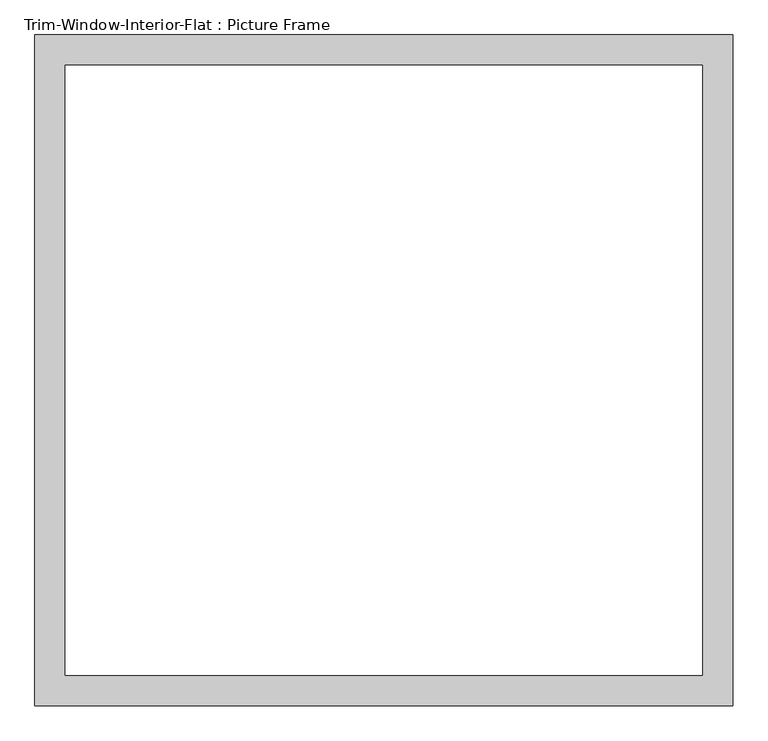
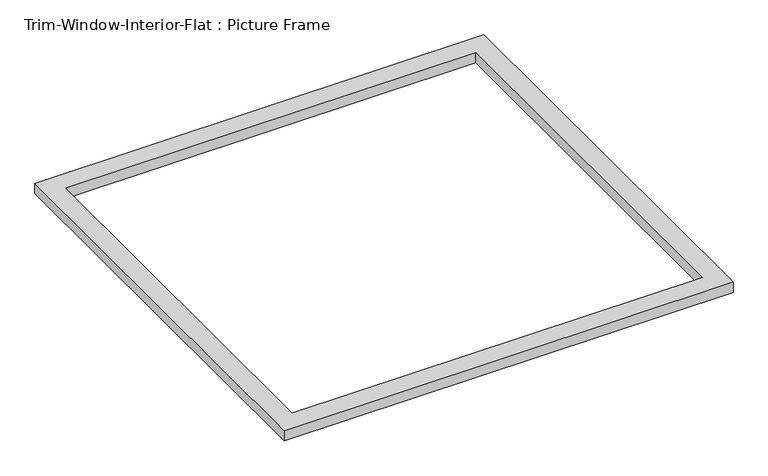
"""IFC4 building model written with IfcOpenShell, lengths in millimetres: proxy geometry, Trim-Window-Interior-Flat : Picture Frame."""

from ifc_helpers import new_model, si_unit, origin, origin_with_axes, place, context, project, spatial, polyline, outline, extrude, source, transform, mapped, element, save


def trim_window_interior_flat_picture_frame_37b958cc(model_context):
    return source(origin(), model_context, "Body", "SweptSolid", [
        extrude(outline(polyline([(654.05, 44.45), (654.05, -1212.85), (-654.05, -1212.85), (-654.05, 44.45), (654.05, 44.45)]), holes=[polyline([(596.9, -12.7), (-596.9, -12.7), (-596.9, -1155.7), (596.9, -1155.7), (596.9, -12.7)])]), origin_with_axes(), (0.0, 0.0, 1.0), 31.75),
    ])


if __name__ == "__main__":
    model = new_model("IFC4")
    model_context = context("Model", 3, world=origin())
    ifc_project = project(units=[si_unit("LENGTHUNIT", "METRE", prefix="MILLI")], contexts=[model_context])
    site = spatial("IfcSite", under=ifc_project)
    building = spatial("IfcBuilding", under=site)
    placement = place(None, origin())
    trim_window_interior_flat_picture_frame_shape = trim_window_interior_flat_picture_frame_37b958cc(model_context)
    element("IfcBuildingElementProxy", 1, Name="Trim-Window-Interior-Flat : Picture Frame", ObjectType="Trim-Window-Interior-Flat : Picture Frame", at=placement, inside=building, context=model_context, shape_type="MappedRepresentation", body=[
        mapped(trim_window_interior_flat_picture_frame_shape, transform((0.0, 0.0, 0.0), x_axis=(1.0, 0.0, 0.0), y_axis=(0.0, 1.0, 0.0), z_axis=(0.0, 0.0, 1.0))),
    ])
    save(model, "model.ifc")

# Revit data of these elements
# Type "Trim-Window-Interior-Flat : Picture Frame"
#   Trim Thickness_Picture Frame = 0' - 1 1/4"
#   Trim Width = 0' - 2 1/4"
#   Trim Thickness_with Sill = 0' - 0 3/4"
#   Sill Thickness = 0' - 1 1/4"
#   Opening Width [instance default] = 2' - 0"
#   Opening Height [instance default] = 3' - 0"
#   Default Elevation = 4' - 0"
#   Sill = no
#   Picture Frame = yes
#   Trim Material [instance default] = none
# Element 1 (IfcBuildingElementProxy, "Trim-Window-Interior-Flat : Picture Frame")
#   Opening Width = 4' - 0"
#   Opening Height = 3' - 10"
#   Trim Material = Wood - Stained
#   Materials on its faces: "Wood - Stained"
# Materials
#   "Wood - Stained": class "Wood", colour RGB 224 178 126, transparency 0, Cost = 0
